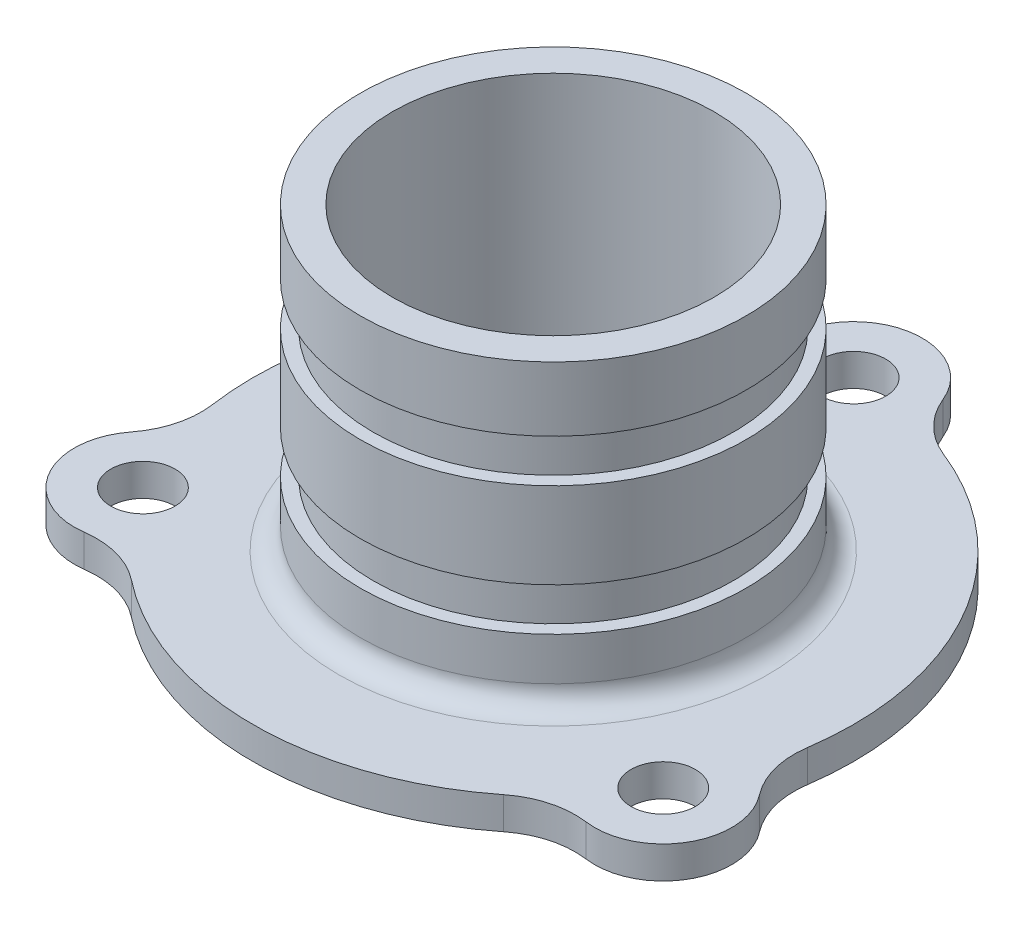
ISO-10303-21;
HEADER;
FILE_DESCRIPTION(('STEP AP214'),'2;1');
FILE_NAME('part.step','',(''),(''),'','','');
FILE_SCHEMA(('AUTOMOTIVE_DESIGN { 1 0 10303 214 1 1 1 1 }'));
ENDSEC;
DATA;
#1=APPLICATION_CONTEXT('core data for automotive mechanical design processes');
#2=APPLICATION_PROTOCOL_DEFINITION('international standard','automotive_design',2000,#1);
#3=PRODUCT_CONTEXT('',#1,'mechanical');
#4=PRODUCT('Part','Part','',(#3));
#5=PRODUCT_RELATED_PRODUCT_CATEGORY('part','',(#4));
#6=PRODUCT_DEFINITION_FORMATION('','',#4);
#7=PRODUCT_DEFINITION_CONTEXT('part definition',#1,'design');
#8=PRODUCT_DEFINITION('design','',#6,#7);
#9=PRODUCT_DEFINITION_SHAPE('','',#8);
#10=(LENGTH_UNIT() NAMED_UNIT(*) SI_UNIT(.MILLI.,.METRE.));
#11=(NAMED_UNIT(*) PLANE_ANGLE_UNIT() SI_UNIT($,.RADIAN.));
#12=(NAMED_UNIT(*) SI_UNIT($,.STERADIAN.) SOLID_ANGLE_UNIT());
#13=UNCERTAINTY_MEASURE_WITH_UNIT(LENGTH_MEASURE(1.E-05),#10,'distance_accuracy_value','');
#14=(GEOMETRIC_REPRESENTATION_CONTEXT(3) GLOBAL_UNCERTAINTY_ASSIGNED_CONTEXT((#13)) GLOBAL_UNIT_ASSIGNED_CONTEXT((#10,
#11,#12)) REPRESENTATION_CONTEXT('',''));
#15=CARTESIAN_POINT('',(0.,0.,0.));
#16=DIRECTION('',(0.,0.,1.));
#17=DIRECTION('',(1.,0.,0.));
#18=AXIS2_PLACEMENT_3D('',#15,#16,#17);
#19=CARTESIAN_POINT('',(0.,41.9950390134529,0.));
#20=DIRECTION('',(0.,1.,0.));
#21=DIRECTION('',(0.,0.,1.));
#22=AXIS2_PLACEMENT_3D('',#19,#20,#21);
#23=PLANE('',#22);
#24=CARTESIAN_POINT('',(0.,41.9950390134529,0.));
#25=DIRECTION('',(0.,1.,0.));
#26=DIRECTION('',(0.,0.,1.));
#27=AXIS2_PLACEMENT_3D('',#24,#25,#26);
#28=CIRCLE('',#27,37.5);
#29=CARTESIAN_POINT('',(0.,41.9950390134529,37.5));
#30=VERTEX_POINT('',#29);
#31=EDGE_CURVE('E224',#30,#30,#28,.T.);
#32=ORIENTED_EDGE('',*,*,#31,.F.);
#33=EDGE_LOOP('',(#32));
#34=FACE_BOUND('',#33,.T.);
#35=CARTESIAN_POINT('',(0.,41.9950390134529,0.));
#36=DIRECTION('',(0.,1.,0.));
#37=DIRECTION('',(0.,0.,1.));
#38=AXIS2_PLACEMENT_3D('',#35,#36,#37);
#39=CIRCLE('',#38,45.);
#40=CARTESIAN_POINT('',(0.,41.9950390134529,45.));
#41=VERTEX_POINT('',#40);
#42=EDGE_CURVE('E244',#41,#41,#39,.T.);
#43=ORIENTED_EDGE('',*,*,#42,.T.);
#44=EDGE_LOOP('',(#43));
#45=FACE_BOUND('',#44,.T.);
#46=ADVANCED_FACE('F41',(#34,#45),#23,.T.);
#47=CARTESIAN_POINT('',(0.,45.6053811659193,0.));
#48=DIRECTION('',(0.,1.,0.));
#49=DIRECTION('',(0.,0.,1.));
#50=AXIS2_PLACEMENT_3D('',#47,#48,#49);
#51=CYLINDRICAL_SURFACE('',#50,45.);
#52=CARTESIAN_POINT('',(0.,26.9950390134529,0.));
#53=DIRECTION('',(0.,1.,0.));
#54=DIRECTION('',(0.,0.,1.));
#55=AXIS2_PLACEMENT_3D('',#52,#53,#54);
#56=CIRCLE('',#55,45.);
#57=CARTESIAN_POINT('',(0.,26.9950390134529,45.));
#58=VERTEX_POINT('',#57);
#59=EDGE_CURVE('E245',#58,#58,#56,.T.);
#60=ORIENTED_EDGE('',*,*,#59,.T.);
#61=EDGE_LOOP('',(#60));
#62=FACE_BOUND('',#61,.T.);
#63=ORIENTED_EDGE('',*,*,#42,.F.);
#64=EDGE_LOOP('',(#63));
#65=FACE_BOUND('',#64,.T.);
#66=ADVANCED_FACE('F262',(#62,#65),#51,.T.);
#67=CARTESIAN_POINT('',(0.,26.9950390134529,0.));
#68=DIRECTION('',(0.,-1.,0.));
#69=DIRECTION('',(0.,0.,-1.));
#70=AXIS2_PLACEMENT_3D('',#67,#68,#69);
#71=PLANE('',#70);
#72=CARTESIAN_POINT('',(0.,26.9950390134529,0.));
#73=DIRECTION('',(0.,1.,0.));
#74=DIRECTION('',(0.,0.,1.));
#75=AXIS2_PLACEMENT_3D('',#72,#73,#74);
#76=CIRCLE('',#75,42.);
#77=CARTESIAN_POINT('',(0.,26.9950390134529,42.));
#78=VERTEX_POINT('',#77);
#79=EDGE_CURVE('E237',#78,#78,#76,.T.);
#80=ORIENTED_EDGE('',*,*,#79,.T.);
#81=EDGE_LOOP('',(#80));
#82=FACE_BOUND('',#81,.T.);
#83=ORIENTED_EDGE('',*,*,#59,.F.);
#84=EDGE_LOOP('',(#83));
#85=FACE_BOUND('',#84,.T.);
#86=ADVANCED_FACE('F275',(#82,#85),#71,.T.);
#87=CARTESIAN_POINT('',(0.,45.6053811659193,0.));
#88=DIRECTION('',(0.,1.,0.));
#89=DIRECTION('',(0.,0.,1.));
#90=AXIS2_PLACEMENT_3D('',#87,#88,#89);
#91=CYLINDRICAL_SURFACE('',#90,42.);
#92=CARTESIAN_POINT('',(0.,16.9950390134529,0.));
#93=DIRECTION('',(0.,1.,0.));
#94=DIRECTION('',(0.,0.,1.));
#95=AXIS2_PLACEMENT_3D('',#92,#93,#94);
#96=CIRCLE('',#95,42.);
#97=CARTESIAN_POINT('',(0.,16.9950390134529,42.));
#98=VERTEX_POINT('',#97);
#99=EDGE_CURVE('E236',#98,#98,#96,.T.);
#100=ORIENTED_EDGE('',*,*,#99,.T.);
#101=EDGE_LOOP('',(#100));
#102=FACE_BOUND('',#101,.T.);
#103=ORIENTED_EDGE('',*,*,#79,.F.);
#104=EDGE_LOOP('',(#103));
#105=FACE_BOUND('',#104,.T.);
#106=ADVANCED_FACE('F278',(#102,#105),#91,.T.);
#107=CARTESIAN_POINT('',(0.,16.9950390134529,0.));
#108=DIRECTION('',(0.,1.,0.));
#109=DIRECTION('',(0.,0.,1.));
#110=AXIS2_PLACEMENT_3D('',#107,#108,#109);
#111=PLANE('',#110);
#112=CARTESIAN_POINT('',(0.,16.9950390134529,0.));
#113=DIRECTION('',(0.,1.,0.));
#114=DIRECTION('',(0.,0.,1.));
#115=AXIS2_PLACEMENT_3D('',#112,#113,#114);
#116=CIRCLE('',#115,45.);
#117=CARTESIAN_POINT('',(0.,16.9950390134529,45.));
#118=VERTEX_POINT('',#117);
#119=EDGE_CURVE('E231',#118,#118,#116,.T.);
#120=ORIENTED_EDGE('',*,*,#119,.T.);
#121=EDGE_LOOP('',(#120));
#122=FACE_BOUND('',#121,.T.);
#123=ORIENTED_EDGE('',*,*,#99,.F.);
#124=EDGE_LOOP('',(#123));
#125=FACE_BOUND('',#124,.T.);
#126=ADVANCED_FACE('F284',(#122,#125),#111,.T.);
#127=CARTESIAN_POINT('',(0.,45.6053811659193,0.));
#128=DIRECTION('',(0.,1.,0.));
#129=DIRECTION('',(0.,0.,1.));
#130=AXIS2_PLACEMENT_3D('',#127,#128,#129);
#131=CYLINDRICAL_SURFACE('',#130,45.);
#132=CARTESIAN_POINT('',(0.,-3.0049609865471,0.));
#133=DIRECTION('',(0.,1.,0.));
#134=DIRECTION('',(0.,0.,1.));
#135=AXIS2_PLACEMENT_3D('',#132,#133,#134);
#136=CIRCLE('',#135,45.);
#137=CARTESIAN_POINT('',(0.,-3.0049609865471,45.));
#138=VERTEX_POINT('',#137);
#139=EDGE_CURVE('E229',#138,#138,#136,.T.);
#140=ORIENTED_EDGE('',*,*,#139,.T.);
#141=EDGE_LOOP('',(#140));
#142=FACE_BOUND('',#141,.T.);
#143=ORIENTED_EDGE('',*,*,#119,.F.);
#144=EDGE_LOOP('',(#143));
#145=FACE_BOUND('',#144,.T.);
#146=ADVANCED_FACE('F287',(#142,#145),#131,.T.);
#147=CARTESIAN_POINT('',(0.,-3.00496098654709,0.));
#148=DIRECTION('',(0.,-1.,0.));
#149=DIRECTION('',(0.,0.,-1.));
#150=AXIS2_PLACEMENT_3D('',#147,#148,#149);
#151=PLANE('',#150);
#152=CARTESIAN_POINT('',(0.,-3.00496098654709,0.));
#153=DIRECTION('',(0.,1.,0.));
#154=DIRECTION('',(0.,0.,1.));
#155=AXIS2_PLACEMENT_3D('',#152,#153,#154);
#156=CIRCLE('',#155,42.);
#157=CARTESIAN_POINT('',(0.,-3.00496098654709,42.));
#158=VERTEX_POINT('',#157);
#159=EDGE_CURVE('E221',#158,#158,#156,.T.);
#160=ORIENTED_EDGE('',*,*,#159,.T.);
#161=EDGE_LOOP('',(#160));
#162=FACE_BOUND('',#161,.T.);
#163=ORIENTED_EDGE('',*,*,#139,.F.);
#164=EDGE_LOOP('',(#163));
#165=FACE_BOUND('',#164,.T.);
#166=ADVANCED_FACE('F292',(#162,#165),#151,.T.);
#167=CARTESIAN_POINT('',(0.,45.6053811659193,0.));
#168=DIRECTION('',(0.,1.,0.));
#169=DIRECTION('',(0.,0.,1.));
#170=AXIS2_PLACEMENT_3D('',#167,#168,#169);
#171=CYLINDRICAL_SURFACE('',#170,42.);
#172=CARTESIAN_POINT('',(0.,-13.0049609865471,0.));
#173=DIRECTION('',(0.,1.,0.));
#174=DIRECTION('',(0.,0.,1.));
#175=AXIS2_PLACEMENT_3D('',#172,#173,#174);
#176=CIRCLE('',#175,42.);
#177=CARTESIAN_POINT('',(0.,-13.0049609865471,42.));
#178=VERTEX_POINT('',#177);
#179=EDGE_CURVE('E223',#178,#178,#176,.T.);
#180=ORIENTED_EDGE('',*,*,#179,.T.);
#181=EDGE_LOOP('',(#180));
#182=FACE_BOUND('',#181,.T.);
#183=ORIENTED_EDGE('',*,*,#159,.F.);
#184=EDGE_LOOP('',(#183));
#185=FACE_BOUND('',#184,.T.);
#186=ADVANCED_FACE('F298',(#182,#185),#171,.T.);
#187=CARTESIAN_POINT('',(0.,-13.0049609865471,0.));
#188=DIRECTION('',(0.,1.,0.));
#189=DIRECTION('',(0.,0.,1.));
#190=AXIS2_PLACEMENT_3D('',#187,#188,#189);
#191=CYLINDRICAL_SURFACE('',#190,37.5);
#192=ORIENTED_EDGE('',*,*,#31,.T.);
#193=EDGE_LOOP('',(#192));
#194=FACE_BOUND('',#193,.T.);
#195=CARTESIAN_POINT('',(0.,-35.5,0.));
#196=DIRECTION('',(0.,1.,0.));
#197=DIRECTION('',(0.,0.,1.));
#198=AXIS2_PLACEMENT_3D('',#195,#196,#197);
#199=CIRCLE('',#198,37.5);
#200=CARTESIAN_POINT('',(0.,-35.5,37.5));
#201=VERTEX_POINT('',#200);
#202=EDGE_CURVE('E421',#201,#201,#199,.T.);
#203=ORIENTED_EDGE('',*,*,#202,.F.);
#204=EDGE_LOOP('',(#203));
#205=FACE_BOUND('',#204,.T.);
#206=ADVANCED_FACE('F299',(#194,#205),#191,.F.);
#207=CARTESIAN_POINT('',(0.,0.,0.));
#208=DIRECTION('',(0.,1.,0.));
#209=DIRECTION('',(0.,0.,1.));
#210=AXIS2_PLACEMENT_3D('',#207,#208,#209);
#211=CYLINDRICAL_SURFACE('',#210,45.);
#212=CARTESIAN_POINT('',(0.,-23.,0.));
#213=DIRECTION('',(0.,1.,0.));
#214=DIRECTION('',(0.,0.,1.));
#215=AXIS2_PLACEMENT_3D('',#212,#213,#214);
#216=CIRCLE('',#215,45.);
#217=CARTESIAN_POINT('',(0.,-23.,45.));
#218=VERTEX_POINT('',#217);
#219=EDGE_CURVE('E49',#218,#218,#216,.T.);
#220=ORIENTED_EDGE('',*,*,#219,.T.);
#221=EDGE_LOOP('',(#220));
#222=FACE_BOUND('',#221,.T.);
#223=CARTESIAN_POINT('',(0.,-13.0049609865471,0.));
#224=DIRECTION('',(0.,1.,0.));
#225=DIRECTION('',(0.,0.,1.));
#226=AXIS2_PLACEMENT_3D('',#223,#224,#225);
#227=CIRCLE('',#226,45.);
#228=CARTESIAN_POINT('',(0.,-13.0049609865471,45.));
#229=VERTEX_POINT('',#228);
#230=EDGE_CURVE('E203',#229,#229,#227,.T.);
#231=ORIENTED_EDGE('',*,*,#230,.F.);
#232=EDGE_LOOP('',(#231));
#233=FACE_BOUND('',#232,.T.);
#234=ADVANCED_FACE('F249',(#222,#233),#211,.T.);
#235=CARTESIAN_POINT('',(0.,-13.0049609865471,0.));
#236=DIRECTION('',(0.,-1.,0.));
#237=DIRECTION('',(0.,0.,-1.));
#238=AXIS2_PLACEMENT_3D('',#235,#236,#237);
#239=PLANE('',#238);
#240=ORIENTED_EDGE('',*,*,#179,.F.);
#241=EDGE_LOOP('',(#240));
#242=FACE_BOUND('',#241,.T.);
#243=ORIENTED_EDGE('',*,*,#230,.T.);
#244=EDGE_LOOP('',(#243));
#245=FACE_BOUND('',#244,.T.);
#246=ADVANCED_FACE('F302',(#242,#245),#239,.F.);
#247=CARTESIAN_POINT('',(33.3304024132271,-35.5,-83.654568165596));
#248=DIRECTION('',(0.,1.,0.));
#249=DIRECTION('',(0.,0.,1.));
#250=AXIS2_PLACEMENT_3D('',#247,#248,#249);
#251=CYLINDRICAL_SURFACE('',#250,20.);
#252=CARTESIAN_POINT('',(33.3304024132271,-28.,-83.654568165596));
#253=DIRECTION('',(0.,-1.,0.));
#254=DIRECTION('',(0.,0.,1.));
#255=AXIS2_PLACEMENT_3D('',#252,#253,#254);
#256=CIRCLE('',#255,20.);
#257=CARTESIAN_POINT('',(25.9277589011278,-28.,-65.0749861188228));
#258=VERTEX_POINT('',#257);
#259=CARTESIAN_POINT('',(14.8135121836565,-28.,-76.0964747402649));
#260=VERTEX_POINT('',#259);
#261=EDGE_CURVE('E164',#258,#260,#256,.T.);
#262=ORIENTED_EDGE('',*,*,#261,.F.);
#263=DIRECTION('',(0.,1.,0.));
#264=VECTOR('',#263,1.);
#265=CARTESIAN_POINT('',(25.9277589011278,-35.5,-65.0749861188228));
#266=LINE('',#265,#264);
#267=CARTESIAN_POINT('',(25.9277589011278,-35.5,-65.0749861188228));
#268=VERTEX_POINT('',#267);
#269=EDGE_CURVE('E59',#268,#258,#266,.T.);
#270=ORIENTED_EDGE('',*,*,#269,.F.);
#271=CARTESIAN_POINT('',(33.3304024132271,-35.5,-83.654568165596));
#272=DIRECTION('',(0.,-1.,0.));
#273=DIRECTION('',(0.,0.,1.));
#274=AXIS2_PLACEMENT_3D('',#271,#272,#273);
#275=CIRCLE('',#274,20.);
#276=CARTESIAN_POINT('',(14.8135121836565,-35.5,-76.0964747402649));
#277=VERTEX_POINT('',#276);
#278=EDGE_CURVE('E199',#268,#277,#275,.T.);
#279=ORIENTED_EDGE('',*,*,#278,.T.);
#280=DIRECTION('',(0.,1.,0.));
#281=VECTOR('',#280,1.);
#282=CARTESIAN_POINT('',(14.8135121836565,-35.5,-76.0964747402649));
#283=LINE('',#282,#281);
#284=EDGE_CURVE('E111',#277,#260,#283,.T.);
#285=ORIENTED_EDGE('',*,*,#284,.T.);
#286=EDGE_LOOP('',(#262,#270,#279,#285));
#287=FACE_BOUND('',#286,.T.);
#288=ADVANCED_FACE('F306',(#287),#251,.F.);
#289=CARTESIAN_POINT('',(0.,-35.5,0.));
#290=DIRECTION('',(0.,1.,0.));
#291=DIRECTION('',(0.,0.,1.));
#292=AXIS2_PLACEMENT_3D('',#289,#290,#291);
#293=CYLINDRICAL_SURFACE('',#292,70.05);
#294=CARTESIAN_POINT('',(0.,-28.,0.));
#295=DIRECTION('',(0.,1.,0.));
#296=DIRECTION('',(0.,0.,1.));
#297=AXIS2_PLACEMENT_3D('',#294,#295,#296);
#298=CIRCLE('',#297,70.05);
#299=CARTESIAN_POINT('',(69.3204705803842,-28.,10.083395187837));
#300=VERTEX_POINT('',#299);
#301=EDGE_CURVE('E198',#300,#258,#298,.T.);
#302=ORIENTED_EDGE('',*,*,#301,.F.);
#303=DIRECTION('',(0.,1.,0.));
#304=VECTOR('',#303,1.);
#305=CARTESIAN_POINT('',(69.3204705803842,-35.5,10.083395187837));
#306=LINE('',#305,#304);
#307=CARTESIAN_POINT('',(69.3204705803842,-35.5,10.083395187837));
#308=VERTEX_POINT('',#307);
#309=EDGE_CURVE('E100',#308,#300,#306,.T.);
#310=ORIENTED_EDGE('',*,*,#309,.F.);
#311=CARTESIAN_POINT('',(0.,-35.5,0.));
#312=DIRECTION('',(0.,1.,0.));
#313=DIRECTION('',(0.,0.,1.));
#314=AXIS2_PLACEMENT_3D('',#311,#312,#313);
#315=CIRCLE('',#314,70.05);
#316=EDGE_CURVE('E152',#308,#268,#315,.T.);
#317=ORIENTED_EDGE('',*,*,#316,.T.);
#318=ORIENTED_EDGE('',*,*,#269,.T.);
#319=EDGE_LOOP('',(#302,#310,#317,#318));
#320=FACE_BOUND('',#319,.T.);
#321=ADVANCED_FACE('F315',(#320),#293,.T.);
#322=CARTESIAN_POINT('',(89.1121823806366,-35.5,12.9623088745856));
#323=DIRECTION('',(0.,1.,0.));
#324=DIRECTION('',(0.,0.,1.));
#325=AXIS2_PLACEMENT_3D('',#322,#323,#324);
#326=CYLINDRICAL_SURFACE('',#325,20.);
#327=CARTESIAN_POINT('',(89.1121823806366,-28.,12.9623088745856));
#328=DIRECTION('',(0.,-1.,0.));
#329=DIRECTION('',(0.,0.,-1.));
#330=AXIS2_PLACEMENT_3D('',#327,#328,#329);
#331=CIRCLE('',#330,20.);
#332=CARTESIAN_POINT('',(73.3082363553385,-28.,25.2193594998159));
#333=VERTEX_POINT('',#332);
#334=EDGE_CURVE('E145',#333,#300,#331,.T.);
#335=ORIENTED_EDGE('',*,*,#334,.F.);
#336=DIRECTION('',(0.,1.,0.));
#337=VECTOR('',#336,1.);
#338=CARTESIAN_POINT('',(73.3082363553385,-35.5,25.2193594998159));
#339=LINE('',#338,#337);
#340=CARTESIAN_POINT('',(73.3082363553385,-35.5,25.2193594998159));
#341=VERTEX_POINT('',#340);
#342=EDGE_CURVE('E139',#341,#333,#339,.T.);
#343=ORIENTED_EDGE('',*,*,#342,.F.);
#344=CARTESIAN_POINT('',(89.1121823806366,-35.5,12.9623088745856));
#345=DIRECTION('',(0.,-1.,0.));
#346=DIRECTION('',(0.,0.,-1.));
#347=AXIS2_PLACEMENT_3D('',#344,#345,#346);
#348=CIRCLE('',#347,20.);
#349=EDGE_CURVE('E136',#341,#308,#348,.T.);
#350=ORIENTED_EDGE('',*,*,#349,.T.);
#351=ORIENTED_EDGE('',*,*,#309,.T.);
#352=EDGE_LOOP('',(#335,#343,#350,#351));
#353=FACE_BOUND('',#352,.T.);
#354=ADVANCED_FACE('F140',(#353),#326,.F.);
#355=CARTESIAN_POINT('',(60.6650795350999,-35.5,35.025));
#356=DIRECTION('',(0.,1.,0.));
#357=DIRECTION('',(0.,0.,1.));
#358=AXIS2_PLACEMENT_3D('',#355,#356,#357);
#359=CYLINDRICAL_SURFACE('',#358,15.9999999999998);
#360=CARTESIAN_POINT('',(60.6650795350999,-28.,35.025));
#361=DIRECTION('',(0.,1.,0.));
#362=DIRECTION('',(0.,0.,1.));
#363=AXIS2_PLACEMENT_3D('',#360,#361,#362);
#364=CIRCLE('',#363,15.9999999999998);
#365=CARTESIAN_POINT('',(58.494724171682,-28.,50.8771152404494));
#366=VERTEX_POINT('',#365);
#367=EDGE_CURVE('E194',#366,#333,#364,.T.);
#368=ORIENTED_EDGE('',*,*,#367,.F.);
#369=DIRECTION('',(0.,1.,0.));
#370=VECTOR('',#369,1.);
#371=CARTESIAN_POINT('',(58.494724171682,-35.5,50.8771152404494));
#372=LINE('',#371,#370);
#373=CARTESIAN_POINT('',(58.494724171682,-35.5,50.8771152404494));
#374=VERTEX_POINT('',#373);
#375=EDGE_CURVE('E150',#374,#366,#372,.T.);
#376=ORIENTED_EDGE('',*,*,#375,.F.);
#377=CARTESIAN_POINT('',(60.6650795350999,-35.5,35.025));
#378=DIRECTION('',(0.,1.,0.));
#379=DIRECTION('',(0.,0.,1.));
#380=AXIS2_PLACEMENT_3D('',#377,#378,#379);
#381=CIRCLE('',#380,15.9999999999998);
#382=EDGE_CURVE('E151',#374,#341,#381,.T.);
#383=ORIENTED_EDGE('',*,*,#382,.T.);
#384=ORIENTED_EDGE('',*,*,#342,.T.);
#385=EDGE_LOOP('',(#368,#376,#383,#384));
#386=FACE_BOUND('',#385,.T.);
#387=ADVANCED_FACE('F159',(#386),#359,.T.);
#388=CARTESIAN_POINT('',(55.7817799674093,-35.5,70.6922592910111));
#389=DIRECTION('',(0.,1.,0.));
#390=DIRECTION('',(0.,0.,1.));
#391=AXIS2_PLACEMENT_3D('',#388,#389,#390);
#392=CYLINDRICAL_SURFACE('',#391,20.0000000000002);
#393=CARTESIAN_POINT('',(55.7817799674093,-28.,70.6922592910111));
#394=DIRECTION('',(0.,-1.,0.));
#395=DIRECTION('',(0.,0.,1.));
#396=AXIS2_PLACEMENT_3D('',#393,#394,#395);
#397=CIRCLE('',#396,20.0000000000002);
#398=CARTESIAN_POINT('',(43.3927116792562,-28.,54.9915909309864));
#399=VERTEX_POINT('',#398);
#400=EDGE_CURVE('E188',#399,#366,#397,.T.);
#401=ORIENTED_EDGE('',*,*,#400,.F.);
#402=DIRECTION('',(0.,1.,0.));
#403=VECTOR('',#402,1.);
#404=CARTESIAN_POINT('',(43.3927116792562,-35.5,54.9915909309864));
#405=LINE('',#404,#403);
#406=CARTESIAN_POINT('',(43.3927116792562,-35.5,54.9915909309864));
#407=VERTEX_POINT('',#406);
#408=EDGE_CURVE('E205',#407,#399,#405,.T.);
#409=ORIENTED_EDGE('',*,*,#408,.F.);
#410=CARTESIAN_POINT('',(55.7817799674093,-35.5,70.6922592910111));
#411=DIRECTION('',(0.,-1.,0.));
#412=DIRECTION('',(0.,0.,1.));
#413=AXIS2_PLACEMENT_3D('',#410,#411,#412);
#414=CIRCLE('',#413,20.0000000000002);
#415=EDGE_CURVE('E157',#407,#374,#414,.T.);
#416=ORIENTED_EDGE('',*,*,#415,.T.);
#417=ORIENTED_EDGE('',*,*,#375,.T.);
#418=EDGE_LOOP('',(#401,#409,#416,#417));
#419=FACE_BOUND('',#418,.T.);
#420=ADVANCED_FACE('F339',(#419),#392,.F.);
#421=CARTESIAN_POINT('',(0.,-35.5,0.));
#422=DIRECTION('',(0.,1.,0.));
#423=DIRECTION('',(0.,0.,1.));
#424=AXIS2_PLACEMENT_3D('',#421,#422,#423);
#425=CYLINDRICAL_SURFACE('',#424,70.05);
#426=CARTESIAN_POINT('',(0.,-28.,0.));
#427=DIRECTION('',(0.,1.,0.));
#428=DIRECTION('',(0.,0.,1.));
#429=AXIS2_PLACEMENT_3D('',#426,#427,#428);
#430=CIRCLE('',#429,70.05);
#431=CARTESIAN_POINT('',(-43.3927116792569,-28.,54.9915909309858));
#432=VERTEX_POINT('',#431);
#433=EDGE_CURVE('E190',#432,#399,#430,.T.);
#434=ORIENTED_EDGE('',*,*,#433,.F.);
#435=DIRECTION('',(0.,1.,0.));
#436=VECTOR('',#435,1.);
#437=CARTESIAN_POINT('',(-43.3927116792569,-35.5,54.9915909309858));
#438=LINE('',#437,#436);
#439=CARTESIAN_POINT('',(-43.3927116792569,-35.5,54.9915909309858));
#440=VERTEX_POINT('',#439);
#441=EDGE_CURVE('E207',#440,#432,#438,.T.);
#442=ORIENTED_EDGE('',*,*,#441,.F.);
#443=CARTESIAN_POINT('',(0.,-35.5,0.));
#444=DIRECTION('',(0.,1.,0.));
#445=DIRECTION('',(0.,0.,1.));
#446=AXIS2_PLACEMENT_3D('',#443,#444,#445);
#447=CIRCLE('',#446,70.05);
#448=EDGE_CURVE('E156',#440,#407,#447,.T.);
#449=ORIENTED_EDGE('',*,*,#448,.T.);
#450=ORIENTED_EDGE('',*,*,#408,.T.);
#451=EDGE_LOOP('',(#434,#442,#449,#450));
#452=FACE_BOUND('',#451,.T.);
#453=ADVANCED_FACE('F331',(#452),#425,.T.);
#454=CARTESIAN_POINT('',(-55.7817799674103,-35.5,70.6922592910103));
#455=DIRECTION('',(0.,1.,0.));
#456=DIRECTION('',(0.,0.,1.));
#457=AXIS2_PLACEMENT_3D('',#454,#455,#456);
#458=CYLINDRICAL_SURFACE('',#457,20.);
#459=CARTESIAN_POINT('',(-55.7817799674103,-28.,70.6922592910103));
#460=DIRECTION('',(0.,-1.,0.));
#461=DIRECTION('',(0.,0.,-1.));
#462=AXIS2_PLACEMENT_3D('',#459,#460,#461);
#463=CIRCLE('',#462,20.);
#464=CARTESIAN_POINT('',(-58.4947241716824,-28.,50.8771152404493));
#465=VERTEX_POINT('',#464);
#466=EDGE_CURVE('E183',#465,#432,#463,.T.);
#467=ORIENTED_EDGE('',*,*,#466,.F.);
#468=DIRECTION('',(0.,1.,0.));
#469=VECTOR('',#468,1.);
#470=CARTESIAN_POINT('',(-58.4947241716824,-35.5,50.8771152404493));
#471=LINE('',#470,#469);
#472=CARTESIAN_POINT('',(-58.4947241716824,-35.5,50.8771152404493));
#473=VERTEX_POINT('',#472);
#474=EDGE_CURVE('E206',#473,#465,#471,.T.);
#475=ORIENTED_EDGE('',*,*,#474,.F.);
#476=CARTESIAN_POINT('',(-55.7817799674103,-35.5,70.6922592910103));
#477=DIRECTION('',(0.,-1.,0.));
#478=DIRECTION('',(0.,0.,-1.));
#479=AXIS2_PLACEMENT_3D('',#476,#477,#478);
#480=CIRCLE('',#479,20.);
#481=EDGE_CURVE('E396',#473,#440,#480,.T.);
#482=ORIENTED_EDGE('',*,*,#481,.T.);
#483=ORIENTED_EDGE('',*,*,#441,.T.);
#484=EDGE_LOOP('',(#467,#475,#482,#483));
#485=FACE_BOUND('',#484,.T.);
#486=ADVANCED_FACE('F333',(#485),#458,.F.);
#487=CARTESIAN_POINT('',(-60.6650795350999,-35.5,35.025));
#488=DIRECTION('',(0.,1.,0.));
#489=DIRECTION('',(0.,0.,1.));
#490=AXIS2_PLACEMENT_3D('',#487,#488,#489);
#491=CYLINDRICAL_SURFACE('',#490,16.);
#492=CARTESIAN_POINT('',(-60.6650795350999,-28.,35.025));
#493=DIRECTION('',(0.,1.,0.));
#494=DIRECTION('',(0.,0.,1.));
#495=AXIS2_PLACEMENT_3D('',#492,#493,#494);
#496=CIRCLE('',#495,16.);
#497=CARTESIAN_POINT('',(-73.3082363553385,-28.,25.2193594998152));
#498=VERTEX_POINT('',#497);
#499=EDGE_CURVE('E181',#498,#465,#496,.T.);
#500=ORIENTED_EDGE('',*,*,#499,.F.);
#501=DIRECTION('',(0.,1.,0.));
#502=VECTOR('',#501,1.);
#503=CARTESIAN_POINT('',(-73.3082363553385,-35.5,25.2193594998152));
#504=LINE('',#503,#502);
#505=CARTESIAN_POINT('',(-73.3082363553385,-35.5,25.2193594998152));
#506=VERTEX_POINT('',#505);
#507=EDGE_CURVE('E208',#506,#498,#504,.T.);
#508=ORIENTED_EDGE('',*,*,#507,.F.);
#509=CARTESIAN_POINT('',(-60.6650795350999,-35.5,35.025));
#510=DIRECTION('',(0.,1.,0.));
#511=DIRECTION('',(0.,0.,1.));
#512=AXIS2_PLACEMENT_3D('',#509,#510,#511);
#513=CIRCLE('',#512,16.);
#514=EDGE_CURVE('E399',#506,#473,#513,.T.);
#515=ORIENTED_EDGE('',*,*,#514,.T.);
#516=ORIENTED_EDGE('',*,*,#474,.T.);
#517=EDGE_LOOP('',(#500,#508,#515,#516));
#518=FACE_BOUND('',#517,.T.);
#519=ADVANCED_FACE('F330',(#518),#491,.T.);
#520=CARTESIAN_POINT('',(-89.1121823806366,-35.5,12.9623088745853));
#521=DIRECTION('',(0.,1.,0.));
#522=DIRECTION('',(0.,0.,1.));
#523=AXIS2_PLACEMENT_3D('',#520,#521,#522);
#524=CYLINDRICAL_SURFACE('',#523,19.9999999999997);
#525=CARTESIAN_POINT('',(-89.1121823806366,-28.,12.9623088745853));
#526=DIRECTION('',(0.,-1.,0.));
#527=DIRECTION('',(0.,0.,1.));
#528=AXIS2_PLACEMENT_3D('',#525,#526,#527);
#529=CIRCLE('',#528,19.9999999999997);
#530=CARTESIAN_POINT('',(-69.3204705803842,-28.,10.0833951878368));
#531=VERTEX_POINT('',#530);
#532=EDGE_CURVE('E178',#531,#498,#529,.T.);
#533=ORIENTED_EDGE('',*,*,#532,.F.);
#534=DIRECTION('',(0.,1.,0.));
#535=VECTOR('',#534,1.);
#536=CARTESIAN_POINT('',(-69.3204705803842,-35.5,10.0833951878368));
#537=LINE('',#536,#535);
#538=CARTESIAN_POINT('',(-69.3204705803842,-35.5,10.0833951878368));
#539=VERTEX_POINT('',#538);
#540=EDGE_CURVE('E215',#539,#531,#537,.T.);
#541=ORIENTED_EDGE('',*,*,#540,.F.);
#542=CARTESIAN_POINT('',(-89.1121823806366,-35.5,12.9623088745853));
#543=DIRECTION('',(0.,-1.,0.));
#544=DIRECTION('',(0.,0.,1.));
#545=AXIS2_PLACEMENT_3D('',#542,#543,#544);
#546=CIRCLE('',#545,19.9999999999997);
#547=EDGE_CURVE('E394',#539,#506,#546,.T.);
#548=ORIENTED_EDGE('',*,*,#547,.T.);
#549=ORIENTED_EDGE('',*,*,#507,.T.);
#550=EDGE_LOOP('',(#533,#541,#548,#549));
#551=FACE_BOUND('',#550,.T.);
#552=ADVANCED_FACE('F324',(#551),#524,.F.);
#553=CARTESIAN_POINT('',(0.,-35.5,0.));
#554=DIRECTION('',(0.,1.,0.));
#555=DIRECTION('',(0.,0.,1.));
#556=AXIS2_PLACEMENT_3D('',#553,#554,#555);
#557=CYLINDRICAL_SURFACE('',#556,70.05);
#558=CARTESIAN_POINT('',(0.,-28.,0.));
#559=DIRECTION('',(0.,1.,0.));
#560=DIRECTION('',(0.,0.,1.));
#561=AXIS2_PLACEMENT_3D('',#558,#559,#560);
#562=CIRCLE('',#561,70.05);
#563=CARTESIAN_POINT('',(-25.9277589011278,-28.,-65.0749861188229));
#564=VERTEX_POINT('',#563);
#565=EDGE_CURVE('E174',#564,#531,#562,.T.);
#566=ORIENTED_EDGE('',*,*,#565,.F.);
#567=DIRECTION('',(0.,1.,0.));
#568=VECTOR('',#567,1.);
#569=CARTESIAN_POINT('',(-25.9277589011278,-35.5,-65.0749861188229));
#570=LINE('',#569,#568);
#571=CARTESIAN_POINT('',(-25.9277589011278,-35.5,-65.0749861188229));
#572=VERTEX_POINT('',#571);
#573=EDGE_CURVE('E211',#572,#564,#570,.T.);
#574=ORIENTED_EDGE('',*,*,#573,.F.);
#575=CARTESIAN_POINT('',(0.,-35.5,0.));
#576=DIRECTION('',(0.,1.,0.));
#577=DIRECTION('',(0.,0.,1.));
#578=AXIS2_PLACEMENT_3D('',#575,#576,#577);
#579=CIRCLE('',#578,70.05);
#580=EDGE_CURVE('E393',#572,#539,#579,.T.);
#581=ORIENTED_EDGE('',*,*,#580,.T.);
#582=ORIENTED_EDGE('',*,*,#540,.T.);
#583=EDGE_LOOP('',(#566,#574,#581,#582));
#584=FACE_BOUND('',#583,.T.);
#585=ADVANCED_FACE('F316',(#584),#557,.T.);
#586=CARTESIAN_POINT('',(-33.330402413227,-35.5,-83.654568165596));
#587=DIRECTION('',(0.,1.,0.));
#588=DIRECTION('',(0.,0.,1.));
#589=AXIS2_PLACEMENT_3D('',#586,#587,#588);
#590=CYLINDRICAL_SURFACE('',#589,20.);
#591=CARTESIAN_POINT('',(-33.330402413227,-28.,-83.654568165596));
#592=DIRECTION('',(0.,-1.,0.));
#593=DIRECTION('',(0.,0.,-1.));
#594=AXIS2_PLACEMENT_3D('',#591,#592,#593);
#595=CIRCLE('',#594,20.);
#596=CARTESIAN_POINT('',(-14.8135121836565,-28.,-76.0964747402649));
#597=VERTEX_POINT('',#596);
#598=EDGE_CURVE('E175',#597,#564,#595,.T.);
#599=ORIENTED_EDGE('',*,*,#598,.F.);
#600=DIRECTION('',(0.,1.,0.));
#601=VECTOR('',#600,1.);
#602=CARTESIAN_POINT('',(-14.8135121836565,-35.5,-76.0964747402649));
#603=LINE('',#602,#601);
#604=CARTESIAN_POINT('',(-14.8135121836565,-35.5,-76.0964747402649));
#605=VERTEX_POINT('',#604);
#606=EDGE_CURVE('E218',#605,#597,#603,.T.);
#607=ORIENTED_EDGE('',*,*,#606,.F.);
#608=CARTESIAN_POINT('',(-33.330402413227,-35.5,-83.654568165596));
#609=DIRECTION('',(0.,-1.,0.));
#610=DIRECTION('',(0.,0.,-1.));
#611=AXIS2_PLACEMENT_3D('',#608,#609,#610);
#612=CIRCLE('',#611,20.);
#613=EDGE_CURVE('E389',#605,#572,#612,.T.);
#614=ORIENTED_EDGE('',*,*,#613,.T.);
#615=ORIENTED_EDGE('',*,*,#573,.T.);
#616=EDGE_LOOP('',(#599,#607,#614,#615));
#617=FACE_BOUND('',#616,.T.);
#618=ADVANCED_FACE('F317',(#617),#590,.F.);
#619=CARTESIAN_POINT('',(0.,-35.5,-70.05));
#620=DIRECTION('',(0.,1.,0.));
#621=DIRECTION('',(0.,0.,1.));
#622=AXIS2_PLACEMENT_3D('',#619,#620,#621);
#623=CYLINDRICAL_SURFACE('',#622,16.);
#624=CARTESIAN_POINT('',(0.,-28.,-70.05));
#625=DIRECTION('',(0.,1.,0.));
#626=DIRECTION('',(0.,0.,1.));
#627=AXIS2_PLACEMENT_3D('',#624,#625,#626);
#628=CIRCLE('',#627,16.);
#629=EDGE_CURVE('E166',#260,#597,#628,.T.);
#630=ORIENTED_EDGE('',*,*,#629,.F.);
#631=ORIENTED_EDGE('',*,*,#284,.F.);
#632=CARTESIAN_POINT('',(0.,-35.5,-70.05));
#633=DIRECTION('',(0.,1.,0.));
#634=DIRECTION('',(0.,0.,1.));
#635=AXIS2_PLACEMENT_3D('',#632,#633,#634);
#636=CIRCLE('',#635,16.);
#637=EDGE_CURVE('E387',#277,#605,#636,.T.);
#638=ORIENTED_EDGE('',*,*,#637,.T.);
#639=ORIENTED_EDGE('',*,*,#606,.T.);
#640=EDGE_LOOP('',(#630,#631,#638,#639));
#641=FACE_BOUND('',#640,.T.);
#642=ADVANCED_FACE('F312',(#641),#623,.T.);
#643=CARTESIAN_POINT('',(16.6652012066135,-35.5,-41.827284082798));
#644=DIRECTION('',(0.,1.,0.));
#645=DIRECTION('',(0.,0.,1.));
#646=AXIS2_PLACEMENT_3D('',#643,#644,#645);
#647=PLANE('',#646);
#648=ORIENTED_EDGE('',*,*,#202,.T.);
#649=EDGE_LOOP('',(#648));
#650=FACE_BOUND('',#649,.T.);
#651=CARTESIAN_POINT('',(-60.6650795350999,-35.5,35.025));
#652=DIRECTION('',(0.,1.,0.));
#653=DIRECTION('',(0.,0.,1.));
#654=AXIS2_PLACEMENT_3D('',#651,#652,#653);
#655=CIRCLE('',#654,7.50000000000065);
#656=CARTESIAN_POINT('',(-60.6650795350999,-35.5,42.5250000000007));
#657=VERTEX_POINT('',#656);
#658=EDGE_CURVE('E375',#657,#657,#655,.T.);
#659=ORIENTED_EDGE('',*,*,#658,.T.);
#660=EDGE_LOOP('',(#659));
#661=FACE_BOUND('',#660,.T.);
#662=CARTESIAN_POINT('',(60.6650795350999,-35.5,35.025));
#663=DIRECTION('',(0.,1.,0.));
#664=DIRECTION('',(0.,0.,1.));
#665=AXIS2_PLACEMENT_3D('',#662,#663,#664);
#666=CIRCLE('',#665,7.50000000000032);
#667=CARTESIAN_POINT('',(60.6650795350999,-35.5,42.5250000000003));
#668=VERTEX_POINT('',#667);
#669=EDGE_CURVE('E370',#668,#668,#666,.T.);
#670=ORIENTED_EDGE('',*,*,#669,.T.);
#671=EDGE_LOOP('',(#670));
#672=FACE_BOUND('',#671,.T.);
#673=CARTESIAN_POINT('',(0.,-35.5,-70.05));
#674=DIRECTION('',(0.,1.,0.));
#675=DIRECTION('',(0.,0.,1.));
#676=AXIS2_PLACEMENT_3D('',#673,#674,#675);
#677=CIRCLE('',#676,7.5);
#678=CARTESIAN_POINT('',(0.,-35.5,-62.55));
#679=VERTEX_POINT('',#678);
#680=EDGE_CURVE('E169',#679,#679,#677,.T.);
#681=ORIENTED_EDGE('',*,*,#680,.T.);
#682=EDGE_LOOP('',(#681));
#683=FACE_BOUND('',#682,.T.);
#684=ORIENTED_EDGE('',*,*,#278,.F.);
#685=ORIENTED_EDGE('',*,*,#316,.F.);
#686=ORIENTED_EDGE('',*,*,#349,.F.);
#687=ORIENTED_EDGE('',*,*,#382,.F.);
#688=ORIENTED_EDGE('',*,*,#415,.F.);
#689=ORIENTED_EDGE('',*,*,#448,.F.);
#690=ORIENTED_EDGE('',*,*,#481,.F.);
#691=ORIENTED_EDGE('',*,*,#514,.F.);
#692=ORIENTED_EDGE('',*,*,#547,.F.);
#693=ORIENTED_EDGE('',*,*,#580,.F.);
#694=ORIENTED_EDGE('',*,*,#613,.F.);
#695=ORIENTED_EDGE('',*,*,#637,.F.);
#696=EDGE_LOOP('',(#684,#685,#686,#687,#688,#689,#690,#691,#692,#693,#694,#695));
#697=FACE_BOUND('',#696,.T.);
#698=ADVANCED_FACE('F153',(#650,#661,#672,#683,#697),#647,.F.);
#699=CARTESIAN_POINT('',(16.6652012066135,-28.,-41.827284082798));
#700=DIRECTION('',(0.,1.,0.));
#701=DIRECTION('',(0.,0.,1.));
#702=AXIS2_PLACEMENT_3D('',#699,#700,#701);
#703=PLANE('',#702);
#704=CARTESIAN_POINT('',(0.,-28.,0.));
#705=DIRECTION('',(0.,1.,0.));
#706=DIRECTION('',(0.,0.,1.));
#707=AXIS2_PLACEMENT_3D('',#704,#705,#706);
#708=CIRCLE('',#707,50.);
#709=CARTESIAN_POINT('',(0.,-28.,50.));
#710=VERTEX_POINT('',#709);
#711=EDGE_CURVE('E11',#710,#710,#708,.F.);
#712=ORIENTED_EDGE('',*,*,#711,.T.);
#713=EDGE_LOOP('',(#712));
#714=FACE_BOUND('',#713,.T.);
#715=CARTESIAN_POINT('',(-60.6650795350999,-28.,35.025));
#716=DIRECTION('',(0.,1.,0.));
#717=DIRECTION('',(0.,0.,1.));
#718=AXIS2_PLACEMENT_3D('',#715,#716,#717);
#719=CIRCLE('',#718,7.50000000000065);
#720=CARTESIAN_POINT('',(-60.6650795350999,-28.,42.5250000000007));
#721=VERTEX_POINT('',#720);
#722=EDGE_CURVE('E380',#721,#721,#719,.T.);
#723=ORIENTED_EDGE('',*,*,#722,.F.);
#724=EDGE_LOOP('',(#723));
#725=FACE_BOUND('',#724,.T.);
#726=CARTESIAN_POINT('',(60.6650795350999,-28.,35.025));
#727=DIRECTION('',(0.,1.,0.));
#728=DIRECTION('',(0.,0.,1.));
#729=AXIS2_PLACEMENT_3D('',#726,#727,#728);
#730=CIRCLE('',#729,7.50000000000032);
#731=CARTESIAN_POINT('',(60.6650795350999,-28.,42.5250000000003));
#732=VERTEX_POINT('',#731);
#733=EDGE_CURVE('E369',#732,#732,#730,.T.);
#734=ORIENTED_EDGE('',*,*,#733,.F.);
#735=EDGE_LOOP('',(#734));
#736=FACE_BOUND('',#735,.T.);
#737=CARTESIAN_POINT('',(0.,-28.,-70.05));
#738=DIRECTION('',(0.,1.,0.));
#739=DIRECTION('',(0.,0.,1.));
#740=AXIS2_PLACEMENT_3D('',#737,#738,#739);
#741=CIRCLE('',#740,7.5);
#742=CARTESIAN_POINT('',(0.,-28.,-62.55));
#743=VERTEX_POINT('',#742);
#744=EDGE_CURVE('E372',#743,#743,#741,.T.);
#745=ORIENTED_EDGE('',*,*,#744,.F.);
#746=EDGE_LOOP('',(#745));
#747=FACE_BOUND('',#746,.T.);
#748=ORIENTED_EDGE('',*,*,#261,.T.);
#749=ORIENTED_EDGE('',*,*,#629,.T.);
#750=ORIENTED_EDGE('',*,*,#598,.T.);
#751=ORIENTED_EDGE('',*,*,#565,.T.);
#752=ORIENTED_EDGE('',*,*,#532,.T.);
#753=ORIENTED_EDGE('',*,*,#499,.T.);
#754=ORIENTED_EDGE('',*,*,#466,.T.);
#755=ORIENTED_EDGE('',*,*,#433,.T.);
#756=ORIENTED_EDGE('',*,*,#400,.T.);
#757=ORIENTED_EDGE('',*,*,#367,.T.);
#758=ORIENTED_EDGE('',*,*,#334,.T.);
#759=ORIENTED_EDGE('',*,*,#301,.T.);
#760=EDGE_LOOP('',(#748,#749,#750,#751,#752,#753,#754,#755,#756,#757,#758,#759));
#761=FACE_BOUND('',#760,.T.);
#762=ADVANCED_FACE('F347',(#714,#725,#736,#747,#761),#703,.T.);
#763=CARTESIAN_POINT('',(0.,-35.5,-70.05));
#764=DIRECTION('',(0.,1.,0.));
#765=DIRECTION('',(0.,0.,1.));
#766=AXIS2_PLACEMENT_3D('',#763,#764,#765);
#767=CYLINDRICAL_SURFACE('',#766,7.5);
#768=ORIENTED_EDGE('',*,*,#680,.F.);
#769=EDGE_LOOP('',(#768));
#770=FACE_BOUND('',#769,.T.);
#771=ORIENTED_EDGE('',*,*,#744,.T.);
#772=EDGE_LOOP('',(#771));
#773=FACE_BOUND('',#772,.T.);
#774=ADVANCED_FACE('F354',(#770,#773),#767,.F.);
#775=CARTESIAN_POINT('',(60.6650795350999,-35.5,35.025));
#776=DIRECTION('',(0.,1.,0.));
#777=DIRECTION('',(0.,0.,1.));
#778=AXIS2_PLACEMENT_3D('',#775,#776,#777);
#779=CYLINDRICAL_SURFACE('',#778,7.50000000000032);
#780=ORIENTED_EDGE('',*,*,#669,.F.);
#781=EDGE_LOOP('',(#780));
#782=FACE_BOUND('',#781,.T.);
#783=ORIENTED_EDGE('',*,*,#733,.T.);
#784=EDGE_LOOP('',(#783));
#785=FACE_BOUND('',#784,.T.);
#786=ADVANCED_FACE('F258',(#782,#785),#779,.F.);
#787=CARTESIAN_POINT('',(-60.6650795350999,-35.5,35.025));
#788=DIRECTION('',(0.,1.,0.));
#789=DIRECTION('',(0.,0.,1.));
#790=AXIS2_PLACEMENT_3D('',#787,#788,#789);
#791=CYLINDRICAL_SURFACE('',#790,7.50000000000065);
#792=ORIENTED_EDGE('',*,*,#658,.F.);
#793=EDGE_LOOP('',(#792));
#794=FACE_BOUND('',#793,.T.);
#795=ORIENTED_EDGE('',*,*,#722,.T.);
#796=EDGE_LOOP('',(#795));
#797=FACE_BOUND('',#796,.T.);
#798=ADVANCED_FACE('F251',(#794,#797),#791,.F.);
#799=CARTESIAN_POINT('',(0.,-23.,0.));
#800=DIRECTION('',(0.,1.,0.));
#801=DIRECTION('',(0.,0.,1.));
#802=AXIS2_PLACEMENT_3D('',#799,#800,#801);
#803=TOROIDAL_SURFACE('',#802,50.,5.);
#804=ORIENTED_EDGE('',*,*,#711,.F.);
#805=EDGE_LOOP('',(#804));
#806=FACE_BOUND('',#805,.T.);
#807=ORIENTED_EDGE('',*,*,#219,.F.);
#808=EDGE_LOOP('',(#807));
#809=FACE_BOUND('',#808,.T.);
#810=ADVANCED_FACE('F43',(#806,#809),#803,.F.);
#811=CLOSED_SHELL('',(#46,#66,#86,#106,#126,#146,#166,#186,#206,#234,#246,#288,#321,#354,#387,
#420,#453,#486,#519,#552,#585,#618,#642,#698,#762,#774,#786,#798,#810));
#812=MANIFOLD_SOLID_BREP('B2',#811);
#813=ADVANCED_BREP_SHAPE_REPRESENTATION('',(#18,#812),#14);
#814=SHAPE_DEFINITION_REPRESENTATION(#9,#813);
ENDSEC;
END-ISO-10303-21;
